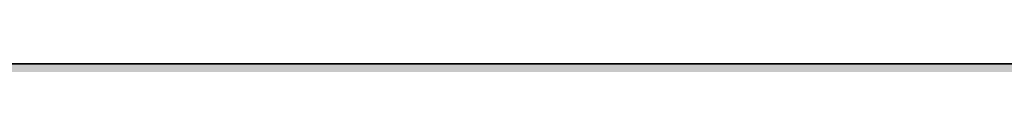
# Model space of a CAD drawing. Units: inches. Extents: x 2091 to 2899, y 967 to 2217.
# Tile 67 of 256: x 2212.646 to 2213.3497, y 1099.9191 to 1099.9191. Entities that reach past the tile are written whole.
import ezdxf

# ---------------------------------------------------------------- set-up
doc = ezdxf.new("R2010")
doc.units = ezdxf.units.IN
doc.layers.add('A-WALL-PATT', color=141, linetype='Continuous', lineweight=13, true_color=0xadddf7)
doc.layers.add('L-SITE-WALL', color=7, linetype='Continuous', lineweight=35)

msp = doc.modelspace()

# ---------------------------------------------------------------- hatches: boundary and pattern name
at = {"layer": 'A-WALL-PATT'}
h = msp.add_hatch(color=256, dxfattribs=at)
h.dxf.hatch_style = 1
h.paths.add_polyline_path([(2212.1436, 1941.41906), (2387.6436, 1941.41906), (2387.6436, 1824.41906), (2392.1436, 1824.41906), (2392.1436, 1941.41906), (2609.6436, 1941.41906), (2609.6436, 1825.91906), (2614.1436, 1825.91906), (2614.1436, 1941.41906), (2794.1436, 1941.41906), (2794.1436, 1928.76217), (2803.1436, 1928.76217), (2803.1436, 2050.91906), (2203.1436, 2050.91906), (2203.1436, 1900.75786), (2212.1436, 1900.75786)])
h.paths.add_polyline_path([(2212.1436, 1945.91906), (2212.1436, 2041.91906), (2794.1436, 2041.91906), (2794.1436, 1945.91906), (2402.24824, 1945.91906), (2401.10243, 1945.77583), (2398.70243, 1945.77583)], flags=16)
h.paths.add_polyline_path([(2230.22986, 1948.06279), (2227.34986, 1949.50279), (2225.90986, 1951.90279), (2223.98986, 1952.86279), (2223.02986, 1955.26279), (2222.06986, 1959.58279), (2222.06986, 1963.42279), (2223.02986, 1965.66279), (2223.98986, 1965.34279), (2225.58591, 1963.86075), (2226.91153, 1964.95726), (2226.94886, 1965.93879), (2227.77832, 1966.95214), (2228.19992, 1968.8787), (2230.70986, 1964.86279), (2233.58986, 1966.30279), (2233.60731, 1966.33187), (2233.77266, 1964.9382), (2234.6338, 1963.67647), (2235.02986, 1963.90279), (2236.28203, 1965.57236), (2235.98986, 1962.94279), (2237.95451, 1957.54), (2238.38986, 1957.90279), (2239.21586, 1960.30579), (2238.65457, 1966.38496), (2238.69279, 1966.43807), (2238.84058, 1967.49971), (2238.78029, 1967.68749), (2238.88054, 1967.78676), (2238.66686, 1966.25179), (2239.21586, 1960.30579), (2238.38986, 1957.90279), (2236.94986, 1956.70279), (2234.54986, 1949.98279)], flags=0)
h.paths.add_polyline_path([(2278.01197, 1948.06279), (2276.49643, 1947.87335), (2275.84983, 1947.68861), (2274.65197, 1947.10279)], flags=0)
h.paths.add_polyline_path([(2269.85197, 1955.74279), (2268.27618, 1956.62933), (2270.8673, 1956.3484), (2269.37197, 1958.14279), (2268.71496, 1959.19233), (2270.56983, 1958.72861), (2268.58073, 1961.90609), (2270.81197, 1960.89188), (2270.81197, 1963.42279), (2271.39331, 1964.77926), (2270.29176, 1966.1562), (2271.77197, 1965.66279), (2272.14139, 1966.52476), (2273.92983, 1965.92861), (2275.63039, 1968.0543), (2276.33194, 1966.72186), (2276.52043, 1966.95214), (2276.94203, 1968.8787), (2277.73429, 1967.61108), (2278.13989, 1969.46452), (2279.65912, 1967.03374), (2280.41197, 1966.78279), (2280.9493, 1967.58879), (2281.60983, 1967.36861), (2282.13327, 1968.15376), (2282.34924, 1966.33344), (2282.34985, 1966.33259), (2283.40755, 1968.09542), (2283.71263, 1965.52402), (2284.32022, 1964.63379), (2284.51181, 1964.88924), (2284.23497, 1965.70479), (2284.50047, 1967.31896), (2284.90794, 1965.41742), (2285.39631, 1966.06858), (2285.43283, 1966.29061), (2285.47334, 1966.17128), (2286.35392, 1967.34539), (2286.22201, 1966.15817), (2287.66349, 1968.08015), (2287.71397, 1968.44279), (2288.4816, 1969.01668), (2288.57399, 1968.7289), (2288.91746, 1969.06904), (2288.60683, 1966.83761), (2288.92873, 1963.35131), (2288.93497, 1963.35679), (2288.92973, 1963.34042), (2289.01528, 1962.41387), (2290.11122, 1963.87513), (2290.13283, 1963.94261), (2290.21767, 1964.01706), (2290.11122, 1963.87513), (2289.15583, 1960.89161), (2288.59404, 1959.25723), (2288.57197, 1959.10279), (2289.53197, 1960.54279), (2290.01197, 1962.46279), (2290.19184, 1962.64266), (2289.76983, 1959.68861), (2286.88983, 1957.28861), (2284.48983, 1950.56861), (2283.31466, 1950.04631), (2283.29197, 1949.98279), (2280.29006, 1948.64861), (2281.12983, 1948.64861), (2282.56983, 1948.16861), (2283.20473, 1948.06279), (2278.97197, 1948.06279), (2276.09197, 1949.50279), (2274.65197, 1951.90279), (2272.73197, 1952.86279)], flags=0)
h.paths.add_polyline_path([(2271.15887, 1958.02177), (2272.96983, 1955.84861), (2272.00983, 1960.16861), (2272.00983, 1964.00861), (2272.62443, 1965.44266), (2274.32802, 1963.86075), (2275.65365, 1964.95726), (2275.63774, 1964.53909), (2277.41223, 1966.00689), (2277.03297, 1965.15679), (2276.82992, 1964.9756), (2276.76601, 1963.29501), (2277.44964, 1962.66022), (2279.45197, 1964.86279), (2282.33197, 1966.30279), (2283.52983, 1966.88861), (2283.29451, 1966.77095), (2283.91299, 1963.8847), (2284.89925, 1964.44827), (2284.73197, 1962.94279), (2286.69662, 1957.54), (2287.13197, 1957.90279), (2287.54191, 1959.09539), (2287.7794, 1958.44231), (2285.68274, 1956.6951), (2285.8765, 1959.79534), (2284.73197, 1962.94279), (2284.89925, 1964.44827), (2283.91299, 1963.8847), (2284.22383, 1962.43412), (2283.42436, 1963.60548), (2281.60983, 1962.56861), (2281.12983, 1960.16861), (2282.08983, 1956.32861), (2283.04983, 1952.96861), (2282.56983, 1950.56861), (2280.16983, 1948.64861), (2279.88332, 1948.79187), (2278.97197, 1948.06279), (2278.97197, 1949.02279), (2278.67231, 1949.39737), (2277.28983, 1950.08861), (2275.84983, 1952.48861), (2273.92983, 1953.44861), (2272.48983, 1954.88861), (2271.92165, 1954.88861), (2271.77197, 1955.26279)], flags=0)
h.paths.add_polyline_path([(2311.99415, 1955.74279), (2312.06272, 1955.67422), (2312.0551, 1955.7085)], flags=0)
h.paths.add_polyline_path([(2331.95615, 1963.95179), (2333.39615, 1965.39179), (2331.07715, 1963.35679), (2330.9986, 1963.11152)], flags=0)
h.paths.add_polyline_path([(2310.55415, 1954.30279), (2307.03981, 1956.27994), (2310.7629, 1955.87628), (2312.47415, 1953.82279), (2313.43415, 1951.42279), (2315.35415, 1950.46279), (2316.79415, 1948.06279), (2317.46615, 1947.72679), (2319.36869, 1947.96461), (2317.75415, 1949.98279), (2317.56953, 1950.61048), (2316.79415, 1951.90279), (2314.87415, 1952.86279), (2313.91415, 1955.26279), (2311.51415, 1958.14279), (2309.37549, 1961.55917), (2311.51415, 1960.33708), (2311.51415, 1961.98279), (2310.60467, 1963.11963), (2311.72661, 1962.47853), (2312.41833, 1964.09256), (2312.25596, 1964.29552), (2313.19415, 1963.98279), (2313.91415, 1965.66279), (2314.64678, 1965.41858), (2315.35415, 1966.30279), (2316.79415, 1967.74279), (2316.15744, 1966.9469), (2317.03411, 1965.28186), (2317.2226, 1965.51214), (2317.77705, 1968.04577), (2318.47411, 1966.72186), (2318.6626, 1966.95214), (2319.0842, 1968.8787), (2321.20705, 1965.48215), (2322.16142, 1966.9137), (2322.55415, 1966.78279), (2322.78599, 1967.13056), (2322.88165, 1966.32429), (2323.31204, 1965.72174), (2323.65129, 1965.89136), (2324.3965, 1967.13338), (2324.65694, 1964.9382), (2324.97199, 1964.47661), (2325.38728, 1967.0015), (2325.94081, 1964.41835), (2327.22893, 1966.13584), (2327.16632, 1965.57236), (2328.05914, 1966.76278), (2328.22458, 1966.24749), (2329.66797, 1967.67691), (2329.66458, 1967.68749), (2329.76482, 1967.78676), (2329.55115, 1966.25179), (2330.10015, 1960.30579), (2329.33281, 1958.07347), (2329.31306, 1957.93523), (2329.63415, 1958.20279), (2330.23415, 1959.10279), (2330.71415, 1961.02279), (2331.03415, 1961.34279), (2330.71415, 1959.10279), (2329.63415, 1958.20279), (2329.27415, 1957.66279), (2327.71211, 1956.3611), (2325.43415, 1949.98279), (2324.33377, 1949.49374), (2323.99415, 1948.54279), (2319.67415, 1946.62279), (2316.79415, 1948.06279), (2315.35415, 1950.46279), (2313.43415, 1951.42279)], flags=0)
h.paths.add_polyline_path([(2321.33568, 1947.95202), (2321.11415, 1948.06279), (2321.11415, 1949.02279), (2319.19415, 1951.42279), (2316.79415, 1959.58279), (2316.66324, 1959.58279), (2315.35415, 1958.14279), (2314.39415, 1958.14279), (2313.1483, 1958.70908), (2312.95415, 1959.58279), (2312.95415, 1960.89188), (2315.83415, 1959.58279), (2316.66324, 1959.58279), (2317.31471, 1960.29941), (2315.0302, 1962.42075), (2316.35582, 1963.51726), (2316.37234, 1963.95162), (2316.4702, 1963.86075), (2317.79582, 1964.95726), (2317.75522, 1963.88969), (2319.17515, 1965.15679), (2319.49841, 1965.88137), (2321.11415, 1965.34279), (2323.23589, 1962.37236), (2325.68635, 1963.77262), (2325.54279, 1962.48058), (2325.19878, 1963.49401), (2324.47851, 1963.08243), (2324.92601, 1960.99412), (2324.07809, 1962.23647), (2322.41479, 1961.28602), (2322.07415, 1959.58279), (2323.03415, 1955.74279), (2323.99415, 1952.38279), (2323.51415, 1949.98279), (2322.14272, 1948.88565), (2322.07415, 1948.54279)], flags=0)
h.paths.add_polyline_path([(2320.20748, 1963.33746), (2320.15415, 1963.42279), (2320.39415, 1963.54279)], flags=0)
h.paths.add_polyline_path([(2353.85053, 1965.8105), (2354.03053, 1965.7505), (2354.33053, 1966.4505), (2354.33053, 1966.9305)], flags=0)
h.paths.add_polyline_path([(2359.02058, 1969.02641), (2359.09838, 1968.90193), (2359.23353, 1969.5195), (2359.23353, 1969.9995)], flags=0)
h.paths.add_polyline_path([(2358.25669, 1966.68167), (2357.9836, 1966.34803), (2358.21127, 1966.14617), (2358.41049, 1966.38957)], flags=0)
h.paths.add_polyline_path([(2357.76847, 1966.05878), (2357.7322, 1965.10497), (2357.75105, 1965.12056), (2357.76953, 1965.6065), (2357.76953, 1966.05784)], flags=0)
h.paths.add_polyline_path([(2359.11153, 1965.3045), (2359.11153, 1964.8245), (2359.84453, 1966.4675), (2359.84453, 1966.9475)], flags=0)
h.paths.add_polyline_path([(2360.22368, 1966.62145), (2360.69853, 1969.3625), (2360.69853, 1969.8425), (2360.21053, 1967.0255), (2360.21053, 1966.6425)], flags=0)
h.paths.add_polyline_path([(2363.45053, 1967.8905), (2363.45053, 1968.3705), (2362.49053, 1966.9305), (2362.65604, 1966.69878)], flags=0)
h.paths.add_polyline_path([(2364.47552, 1966.07883), (2365.85053, 1968.3705), (2365.85053, 1968.8505), (2364.42798, 1966.47958)], flags=0)
h.paths.add_polyline_path([(2366.31353, 1965.8525), (2366.36671, 1965.69583), (2366.80253, 1968.3455), (2366.80253, 1968.8255)], flags=0)
h.paths.add_polyline_path([(2367.16531, 1965.80354), (2367.29053, 1966.9305), (2367.29053, 1967.4105), (2367.1027, 1965.72007)], flags=0)
h.paths.add_polyline_path([(2370.03653, 1959.9735), (2371.01353, 1963.0245), (2371.01353, 1963.5045), (2370.03653, 1960.4535)], flags=0)
h.paths.add_polyline_path([(2371.61053, 1960.2105), (2372.57053, 1961.6505), (2372.57053, 1962.1305), (2371.80253, 1960.9785)], flags=0)
h.paths.add_polyline_path([(2350.87367, 1956.00509), (2351.93053, 1955.8905), (2354.49053, 1953.3305), (2353.85053, 1954.9305), (2351.45053, 1957.8105), (2347.93553, 1963.4255), (2347.93553, 1963.9055), (2351.45053, 1958.2905), (2353.70507, 1955.58505), (2352.89053, 1959.2505), (2352.89053, 1959.7305), (2352.89053, 1961.92479), (2356.73053, 1959.7305), (2358.45447, 1961.62684), (2354.81053, 1965.0105), (2355.03086, 1965.28591), (2358.69109, 1961.88712), (2361.53053, 1965.0105), (2364.3765, 1966.43348), (2364.52439, 1965.18691), (2365.45447, 1963.82418), (2365.88107, 1964.06795), (2365.37053, 1966.4505), (2365.37053, 1966.9305), (2366.81053, 1960.2105), (2366.81053, 1959.7305), (2366.38871, 1952.98141), (2367.77053, 1956.8505), (2368.64123, 1957.57608), (2366.81053, 1962.6105), (2366.81053, 1963.0905), (2368.77518, 1957.68771), (2369.21053, 1958.0505), (2370.00159, 1960.35187), (2369.47523, 1966.05267), (2369.51346, 1966.10578), (2369.51417, 1966.11091), (2369.47523, 1966.53267), (2369.51346, 1966.58578), (2369.61463, 1967.31259), (2369.18253, 1968.6585), (2369.18253, 1969.1385), (2369.60096, 1967.83519), (2369.7012, 1967.93447), (2369.71795, 1968.05474), (2370.14518, 1968.37414), (2369.77871, 1968.01122), (2369.7012, 1967.45447), (2370.46816, 1968.214), (2369.67494, 1967.26577), (2369.51417, 1966.11091), (2370.03653, 1960.4535), (2370.03653, 1959.9735), (2369.44176, 1958.24319), (2370.65053, 1959.2505), (2371.04582, 1962.01756), (2371.13053, 1962.1305), (2370.65053, 1958.7705), (2367.77053, 1956.3705), (2365.37053, 1949.6505), (2362.0791, 1948.18764), (2363.45053, 1947.7305), (2361.05053, 1947.7305), (2360.09053, 1947.7305), (2357.10386, 1947.35717), (2360.09053, 1948.2105), (2358.17053, 1949.1705), (2356.73053, 1951.5705), (2354.81053, 1952.5305), (2351.93053, 1955.4105)], flags=0)
h.paths.add_polyline_path([(2361.05053, 1948.6905), (2359.13053, 1951.0905), (2356.73053, 1959.2505), (2355.77053, 1959.2505), (2352.89053, 1960.55959), (2352.89053, 1961.44479), (2355.89053, 1959.7305), (2356.73053, 1959.7305), (2356.83719, 1959.36783), (2361.53053, 1964.5305), (2363.24842, 1965.38945), (2364.92531, 1963.0418), (2362.49053, 1961.6505), (2362.06386, 1959.51717), (2362.97053, 1955.8905), (2363.93053, 1952.5305), (2363.93053, 1952.0505), (2363.45053, 1949.6505), (2361.05053, 1947.7305)], flags=0)
h.paths.add_polyline_path([(2359.13053, 1951.5705), (2359.29053, 1951.3705), (2361.05053, 1954.4505), (2361.05053, 1954.9305)], flags=0)
h.paths.add_polyline_path([(2357.21953, 1966.5455), (2356.79253, 1968.8145), (2356.79253, 1969.2945), (2357.21953, 1967.0255)], flags=0)
h.paths.add_polyline_path([(2361.05053, 1954.4505), (2361.53053, 1958.7705), (2361.53053, 1959.2505), (2361.05053, 1954.9305)], flags=0)
h.paths.add_polyline_path([(2402.54829, 1948.48608), (2402.30243, 1948.41583), (2402.59043, 1948.41583)], flags=0)
h.paths.add_polyline_path([(2394.14243, 1956.09583), (2395.68505, 1954.55321), (2396.7205, 1953.97068), (2396.06243, 1955.61583), (2395.24138, 1956.6011), (2395.8789, 1956.44171), (2395.10243, 1959.93583), (2395.10243, 1963.77583), (2396.06243, 1966.01583), (2397.02243, 1965.69583), (2398.61848, 1964.21379), (2399.94411, 1965.3103), (2399.98143, 1966.29183), (2400.81089, 1967.30518), (2401.23249, 1969.23174), (2403.53795, 1965.54301), (2403.94198, 1967.38932), (2404.70243, 1967.13583), (2405.46033, 1966.07478), (2406.62243, 1966.65583), (2406.63988, 1966.68491), (2406.80523, 1965.29124), (2406.92569, 1965.11475), (2407.34243, 1964.97583), (2407.87433, 1965.77367), (2408.1691, 1964.39805), (2409.31461, 1965.9254), (2409.21746, 1965.05105), (2409.44523, 1963.13124), (2410.30637, 1961.86951), (2410.70243, 1962.09583), (2411.44227, 1963.08228), (2411.16543, 1963.89783), (2411.61643, 1966.63976), (2411.72536, 1966.79111), (2411.87315, 1967.85275), (2411.81286, 1968.04053), (2411.91311, 1968.1398), (2411.69943, 1966.60483), (2412.24843, 1960.65883), (2413.22543, 1963.70983), (2414.3779, 1964.72116), (2414.51315, 1965.69275), (2414.45286, 1965.88053), (2414.55311, 1965.9798), (2414.3779, 1964.72116), (2414.51982, 1964.8457), (2414.36536, 1964.63111), (2414.33943, 1964.44483), (2414.88843, 1958.49883), (2414.06243, 1956.09583), (2412.62243, 1954.89583), (2410.17137, 1948.03285), (2410.01672, 1948.0844), (2405.90243, 1946.25583), (2405.90243, 1947.21583), (2405.20425, 1948.08856), (2404.22243, 1948.41583), (2403.26243, 1948.41583), (2400.38243, 1949.85583), (2399.66243, 1951.05583), (2397.98243, 1952.73583), (2397.02243, 1953.21583), (2395.68505, 1954.55321), (2392.65678, 1956.25691)], flags=0)
h.paths.add_polyline_path([(2409.08565, 1964.40744), (2409.13036, 1964.27572), (2409.26243, 1964.49583)], flags=0)
h.paths.add_polyline_path([(2397.74243, 1961.61583), (2398.70243, 1963.85583), (2399.66243, 1963.53583), (2401.42656, 1965.74099), (2401.79142, 1966.5588), (2402.07143, 1965.07083), (2402.83551, 1964.39337), (2403.2624, 1964.9149), (2403.33812, 1964.77109), (2402.61552, 1963.97622), (2402.49861, 1960.90224), (2403.543, 1959.93245), (2404.4132, 1960.88968), (2404.70243, 1962.33583), (2407.91635, 1964.17235), (2409.52021, 1961.92694), (2410.98708, 1957.89304), (2411.42243, 1958.25583), (2412.04796, 1960.07562), (2412.41034, 1959.07909), (2411.67562, 1958.46682), (2411.66243, 1958.25583), (2411.62607, 1958.42553), (2409.98243, 1957.05583), (2407.58243, 1950.33583), (2403.26243, 1948.41583), (2403.26243, 1949.37583), (2401.34243, 1951.77583), (2399.41651, 1958.32398), (2397.74243, 1959.08492), (2397.74243, 1959.97012), (2397.10243, 1960.33583), (2397.74243, 1960.04492)], flags=0)
h.paths.add_polyline_path([(2405.90243, 1952.97583), (2405.95043, 1953.40783), (2406.01672, 1953.17583)], flags=0)
h.paths.add_polyline_path([(2449.81778, 1967.11401), (2449.75232, 1967.13583), (2449.7937, 1967.0779)], flags=0)
h.paths.add_polyline_path([(2451.6977, 1966.61812), (2451.74089, 1966.69012), (2451.69205, 1966.6657)], flags=0)
h.paths.add_polyline_path([(2454.34363, 1965.73757), (2455.75232, 1967.61583), (2455.99232, 1968.09583), (2454.3645, 1965.9254)], flags=0)
h.paths.add_polyline_path([(2457.54732, 1968.86383), (2457.78732, 1969.34383), (2457.05432, 1968.79583), (2457.00762, 1968.46034)], flags=0)
h.paths.add_polyline_path([(2456.92178, 1967.85666), (2456.80224, 1968.22902), (2456.723, 1967.6598)], flags=0)
h.paths.add_polyline_path([(2457.30232, 1967.37683), (2457.54232, 1967.85683), (2456.81032, 1966.83983), (2456.74052, 1966.70022), (2456.74902, 1966.60811)], flags=0)
h.paths.add_polyline_path([(2458.27532, 1963.70983), (2458.15534, 1963.33515), (2460.35432, 1965.26483), (2460.59432, 1965.74483)], flags=0)
h.paths.add_polyline_path([(2458.39232, 1962.81583), (2458.36409, 1962.61819), (2459.59232, 1964.25583), (2459.83232, 1964.73583)], flags=0)
h.paths.add_polyline_path([(2459.35232, 1962.81583), (2459.27232, 1962.49583), (2460.07232, 1963.29583), (2460.31232, 1963.77583)], flags=0)
h.paths.add_polyline_path([(2458.68032, 1960.60783), (2458.63232, 1960.41583), (2459.59232, 1961.85583), (2459.83232, 1962.33583)], flags=0)
h.paths.add_polyline_path([(2437.83817, 1956.24265), (2439.19232, 1956.09583), (2441.35232, 1953.93583), (2440.87232, 1955.13583), (2438.47232, 1958.01583), (2438.07156, 1958.65602), (2438.71232, 1958.49583), (2440.6396, 1956.18311), (2439.91232, 1959.45583), (2439.91232, 1963.29583), (2441.35232, 1966.65583), (2441.59232, 1967.13583), (2441.11232, 1966.01583), (2442.07232, 1965.69583), (2443.98899, 1968.09167), (2444.24132, 1966.75083), (2444.9168, 1966.15192), (2445.67657, 1967.08014), (2446.25532, 1969.72483), (2446.49532, 1970.20483), (2446.28238, 1969.23174), (2447.36267, 1967.50327), (2447.72032, 1969.56783), (2447.96032, 1970.04783), (2447.48548, 1967.30678), (2448.79232, 1965.21583), (2448.47232, 1964.86383), (2448.55232, 1964.73583), (2451.45205, 1966.1857), (2451.61512, 1964.81124), (2452.30792, 1963.79617), (2453.23451, 1964.32565), (2454.07232, 1960.41583), (2453.62869, 1953.31765), (2454.79232, 1956.57583), (2455.03232, 1957.05583), (2455.71884, 1957.62793), (2453.83232, 1962.81583), (2453.94097, 1963.79362), (2453.33532, 1965.57783), (2453.82432, 1968.55083), (2454.06432, 1969.03083), (2453.57532, 1966.05783), (2454.04033, 1964.68792), (2453.83232, 1962.81583), (2455.71884, 1957.62793), (2456.36721, 1958.16824), (2457.05832, 1960.17883), (2457.29832, 1960.65883), (2456.47232, 1958.25583), (2457.71773, 1959.29367), (2457.67232, 1958.97583), (2454.88995, 1956.65719), (2453.61414, 1953.08492), (2453.59232, 1952.73583), (2453.35232, 1952.25583), (2453.3596, 1952.3722), (2452.63232, 1950.33583), (2452.39232, 1949.85583), (2449.20375, 1948.43869), (2450.71232, 1947.93583), (2448.07232, 1947.93583), (2447.11232, 1947.93583), (2444.55232, 1947.61583), (2447.1996, 1948.3722), (2445.19232, 1949.37583), (2443.75232, 1951.77583), (2441.83232, 1952.73583), (2438.95232, 1955.61583)], flags=0)
h.paths.add_polyline_path([(2443.99232, 1959.93583), (2444.04032, 1959.77263), (2444.12155, 1959.86199)], flags=0)
h.paths.add_polyline_path([(2442.91232, 1959.93583), (2443.03232, 1959.93583), (2442.44566, 1960.2025)], flags=0)
h.paths.add_polyline_path([(2444.98294, 1965.01968), (2445.27932, 1965.26483), (2445.51932, 1965.74483), (2444.994, 1965.3103)], flags=0)
h.paths.add_polyline_path([(2446.13332, 1965.02983), (2446.33037, 1965.4715), (2444.97032, 1964.25783), (2444.73032, 1963.77783)], flags=0)
h.paths.add_polyline_path([(2442.79232, 1959.45583), (2443.75232, 1959.45583), (2446.15232, 1951.29583), (2446.41232, 1951.75083), (2446.39232, 1951.77583), (2448.0806, 1954.73032), (2448.55232, 1958.97583), (2441.83232, 1965.21583), (2442.15495, 1965.61911), (2448.79232, 1959.45583), (2448.31232, 1955.13583), (2448.07232, 1954.65583), (2446.41232, 1951.75083), (2448.31232, 1949.37583), (2448.31232, 1948.41583), (2450.54089, 1950.19869), (2450.95232, 1952.25583), (2449.99232, 1955.61583), (2449.03232, 1959.45583), (2449.51232, 1961.85583), (2449.75232, 1962.33583), (2449.6749, 1961.94874), (2452.99451, 1963.84565), (2453.06441, 1963.51941), (2452.88461, 1963.78285), (2449.6749, 1961.94874), (2449.27232, 1959.93583), (2450.23232, 1956.09583), (2451.19232, 1952.73583), (2450.71232, 1950.33583), (2450.47232, 1949.85583), (2448.07232, 1947.93583), (2448.07232, 1948.53583), (2445.43232, 1949.85583), (2443.99232, 1952.25583), (2442.07232, 1953.21583), (2441.11232, 1955.61583), (2440.15232, 1959.93583), (2440.15232, 1960.65583)], flags=0)
h.paths.add_polyline_path([(2456.69232, 1966.98583), (2457.60832, 1968.08083), (2457.84832, 1968.56083), (2456.93232, 1967.46583)], flags=0)
h.paths.add_polyline_path([(2489.89657, 1966.58024), (2489.94295, 1966.18935), (2490.74749, 1967.53025), (2491.31912, 1968.95116)], flags=0)
h.paths.add_polyline_path([(2473.56247, 1956.40713), (2477.13998, 1956.01926), (2476.95533, 1956.24083), (2475.10805, 1957.28011), (2476.34749, 1956.97025), (2475.1869, 1958.82422), (2476.91912, 1958.39116), (2475.41164, 1960.79927), (2477.78749, 1959.71934), (2477.78749, 1962.25025), (2477.6374, 1962.43786), (2477.82255, 1962.33206), (2478.35912, 1963.58406), (2478.35912, 1963.67116), (2477.32435, 1964.96463), (2478.71483, 1964.50114), (2479.31912, 1965.91116), (2480.27912, 1965.59116), (2481.78397, 1967.47221), (2482.11649, 1965.70525), (2482.88056, 1965.02778), (2483.20931, 1965.42941), (2483.22017, 1965.71509), (2483.07594, 1965.98902), (2483.71176, 1966.76581), (2484.13049, 1968.67925), (2484.70212, 1970.10016), (2484.48918, 1969.12707), (2486.5029, 1965.90511), (2487.38749, 1965.61025), (2488.15342, 1966.75914), (2488.71702, 1965.97011), (2489.20009, 1966.21164), (2489.33067, 1965.11099), (2490.3939, 1963.62246), (2490.66077, 1963.77496), (2490.49391, 1964.55364), (2490.92306, 1963.92484), (2491.31912, 1964.15116), (2491.33339, 1964.17018), (2491.21049, 1964.53225), (2491.28176, 1964.96554), (2491.42579, 1964.29338), (2494.07648, 1967.82763), (2494.49792, 1966.51494), (2494.59817, 1966.61422), (2494.68949, 1967.27025), (2495.10675, 1967.5822), (2495.12984, 1967.74807), (2495.06955, 1967.93585), (2495.1698, 1968.03513), (2495.03178, 1967.04363), (2495.75382, 1967.75868), (2494.98205, 1966.68644), (2494.95612, 1966.50016), (2495.47902, 1960.83685), (2495.91049, 1962.18425), (2496.48212, 1963.60516), (2496.07269, 1962.32659), (2496.7689, 1962.93754), (2496.59912, 1962.71116), (2496.11912, 1959.35116), (2496.73287, 1960.27179), (2496.98749, 1961.29025), (2497.55912, 1962.71116), (2497.07912, 1960.79116), (2496.50749, 1959.37025), (2495.54749, 1957.93025), (2492.75884, 1955.60638), (2490.83912, 1950.23116), (2490.26749, 1948.81025), (2485.94749, 1946.89025), (2483.06749, 1948.33025), (2481.62749, 1950.73025), (2479.70749, 1951.69025), (2476.82749, 1954.57025)], flags=0)
h.paths.add_polyline_path([(2485.57697, 1948.31339), (2485.55912, 1948.31116), (2485.57876, 1948.31116)], flags=0)
h.paths.add_polyline_path([(2478.64506, 1954.55116), (2478.10904, 1956.96326), (2479.31912, 1955.51116), (2480.27912, 1953.11116), (2482.19912, 1952.15116), (2483.63912, 1949.75116), (2486.51912, 1948.31116), (2486.51912, 1949.27116), (2484.73931, 1951.49593), (2484.02749, 1950.25025), (2481.62749, 1958.41025), (2482.37515, 1959.23267), (2482.19912, 1959.83116), (2483.19757, 1960.92946), (2479.70749, 1964.17025), (2480.60336, 1965.29008), (2481.87517, 1964.10911), (2482.66639, 1964.76358), (2482.61536, 1963.4218), (2482.9892, 1963.07466), (2484.00849, 1963.98425), (2484.68361, 1965.49751), (2484.58012, 1965.40516), (2485.35727, 1967.14711), (2485.12065, 1965.7812), (2486.42749, 1963.69025), (2488.14538, 1964.5492), (2489.82227, 1962.20155), (2490.74749, 1962.73025), (2491.99966, 1964.39981), (2492.07605, 1965.08726), (2492.21289, 1964.68412), (2492.48537, 1965.04743), (2492.27912, 1963.19116), (2494.24377, 1957.78837), (2494.5625, 1958.05398), (2494.93349, 1959.13325), (2495.50512, 1960.55416), (2494.67912, 1958.15116), (2494.10749, 1956.73025), (2494.5625, 1958.05398), (2493.40854, 1957.09235), (2491.70749, 1961.77025), (2491.99966, 1964.39981), (2490.74749, 1962.73025), (2487.71203, 1960.9957), (2487.47912, 1959.83116), (2488.43912, 1955.99116), (2489.39912, 1952.63116), (2488.91912, 1950.23116), (2488.57692, 1949.9574), (2488.34749, 1948.81025), (2487.65172, 1948.25363), (2487.47912, 1948.31116), (2486.51912, 1948.31116), (2483.63912, 1949.75116), (2482.19912, 1952.15116), (2480.27912, 1953.11116), (2478.83912, 1954.55116)], flags=0)
h.paths.add_polyline_path([(2526.64825, 1966.98752), (2526.51734, 1967.03116), (2526.6001, 1966.9153)], flags=0)
h.paths.add_polyline_path([(2528.47064, 1966.44666), (2528.57449, 1966.61973), (2528.45707, 1966.56102)], flags=0)
h.paths.add_polyline_path([(2534.13334, 1967.49616), (2534.15669, 1967.54285), (2534.05984, 1967.4083)], flags=0)
h.paths.add_polyline_path([(2536.16192, 1964.0506), (2535.15734, 1962.71116), (2535.10087, 1962.31587), (2536.11734, 1963.67116), (2536.42053, 1964.27754)], flags=0)
h.paths.add_polyline_path([(2535.15734, 1959.83116), (2536.11734, 1961.27116), (2536.59734, 1962.23116), (2535.25334, 1960.21516)], flags=0)
h.paths.add_polyline_path([(2513.24904, 1956.2848), (2516.22118, 1955.96256), (2514.99734, 1957.43116), (2514.19582, 1958.71154), (2515.47734, 1958.39116), (2516.93189, 1956.64571), (2516.43734, 1958.87116), (2516.43734, 1962.71116), (2516.87269, 1963.72697), (2515.34643, 1965.6348), (2517.39734, 1964.95116), (2517.87734, 1966.07116), (2518.35734, 1967.03116), (2517.87734, 1965.91116), (2518.83734, 1965.59116), (2520.48659, 1967.65272), (2520.76634, 1966.16616), (2521.53042, 1965.48869), (2521.78144, 1965.79537), (2521.80091, 1966.30727), (2521.4778, 1966.92094), (2521.24634, 1967.12616), (2521.1777, 1967.49091), (2521.4778, 1966.92094), (2522.01042, 1966.44869), (2522.25739, 1966.75042), (2522.78034, 1969.14016), (2523.26034, 1970.10016), (2523.0474, 1969.12707), (2524.67313, 1966.5259), (2526.03734, 1966.07116), (2526.79524, 1965.01011), (2527.97707, 1965.60102), (2528.14014, 1964.22657), (2528.66459, 1963.45816), (2529.38862, 1963.87189), (2529.32967, 1964.14699), (2529.48128, 1963.92484), (2529.87734, 1964.15116), (2529.98401, 1964.29338), (2529.78905, 1965.20318), (2530.0624, 1964.3979), (2532.80248, 1968.05135), (2533.14777, 1966.97585), (2533.24802, 1967.07513), (2533.33934, 1967.73116), (2533.67285, 1967.98049), (2533.72802, 1968.03513), (2533.51434, 1966.50016), (2534.02472, 1960.9725), (2534.56034, 1962.64516), (2535.04034, 1963.60516), (2534.06334, 1960.55416), (2533.23734, 1958.15116), (2534.28815, 1959.02684), (2534.19734, 1958.39116), (2531.5126, 1956.15387), (2529.39734, 1950.23116), (2528.91734, 1949.27116), (2526.44877, 1948.17402), (2527.47734, 1947.83116), (2530.35734, 1947.35116), (2524.59734, 1947.35116), (2521.71734, 1948.79116), (2520.27734, 1951.19116), (2518.35734, 1952.15116), (2515.47734, 1955.03116)], flags=0)
h.paths.add_polyline_path([(2523.93476, 1967.19031), (2523.61951, 1966.48369), (2523.7705, 1966.24211)], flags=0)
h.paths.add_polyline_path([(2518.83734, 1953.11116), (2517.87734, 1955.51116), (2516.88498, 1959.97678), (2516.91734, 1959.96207), (2516.91734, 1962.02545), (2520.75734, 1959.83116), (2522.02495, 1961.22553), (2518.35734, 1964.63116), (2519.00259, 1965.43772), (2520.43339, 1964.10911), (2521.30112, 1964.82687), (2521.24516, 1963.35533), (2525.63831, 1959.27598), (2526.03734, 1961.27116), (2529.39734, 1963.19116), (2530.64952, 1964.86073), (2530.66472, 1964.99755), (2530.69196, 1964.91731), (2531.08778, 1965.44507), (2530.94599, 1964.16894), (2530.69196, 1964.91731), (2529.39734, 1963.19116), (2526.3625, 1961.45697), (2526.03734, 1959.83116), (2526.99734, 1955.99116), (2527.95734, 1952.63116), (2527.47734, 1950.23116), (2527.13449, 1949.95687), (2526.97393, 1949.15409), (2526.69734, 1949.03116), (2524.59734, 1947.35116), (2524.59734, 1948.31116), (2524.27734, 1948.71116), (2522.19734, 1949.75116), (2520.75734, 1952.15116)], flags=0)
h.paths.add_polyline_path([(2520.27734, 1958.87116), (2520.85334, 1959.50476), (2523.15734, 1951.67116), (2524.61389, 1954.22013), (2524.59734, 1954.07116), (2522.67734, 1950.71116)], flags=0)
h.paths.add_polyline_path([(2559.37091, 1966.31116), (2559.39841, 1966.32491), (2559.40194, 1966.3453)], flags=0)
h.paths.add_polyline_path([(2549.77091, 1957.19116), (2552.65091, 1954.31116), (2552.13399, 1955.60347), (2550.61091, 1957.43116), (2547.09591, 1963.04616), (2545.77591, 1965.20616), (2549.29091, 1959.59116), (2551.69091, 1956.71116), (2550.79293, 1960.75206), (2550.73091, 1960.78025), (2550.73091, 1964.87116), (2551.69091, 1967.11116), (2552.65091, 1966.79116), (2554.24696, 1965.30911), (2555.03425, 1965.96034), (2555.58167, 1966.64461), (2555.60991, 1967.38716), (2556.43937, 1968.40051), (2556.86097, 1970.32707), (2559.37091, 1966.31116), (2560.69091, 1964.15116), (2562.40881, 1965.01011), (2561.65091, 1966.07116), (2560.33091, 1968.23116), (2561.7585, 1966.23254), (2562.34721, 1967.11561), (2562.43371, 1966.38657), (2563.1278, 1965.3696), (2563.57091, 1965.59116), (2563.58836, 1965.62024), (2563.36254, 1967.52354), (2563.72249, 1965.84379), (2565.06, 1968.07298), (2564.73286, 1965.12872), (2565.11758, 1963.33338), (2567.44462, 1966.43611), (2567.31561, 1967.83333), (2567.35384, 1967.88644), (2567.50163, 1968.94807), (2567.44134, 1969.13585), (2567.54159, 1969.23513), (2567.32791, 1967.70016), (2567.87691, 1961.75416), (2568.74669, 1964.47033), (2568.63561, 1965.67333), (2568.67384, 1965.72644), (2568.82163, 1966.78807), (2568.76134, 1966.97585), (2568.86159, 1967.07513), (2568.64791, 1965.54016), (2568.72613, 1964.69303), (2568.85391, 1964.80516), (2568.74669, 1964.47033), (2568.81724, 1963.70626), (2568.97091, 1963.91116), (2568.86607, 1963.17731), (2569.19691, 1959.59416), (2568.37091, 1957.19116), (2566.93091, 1955.99116), (2564.62027, 1949.52137), (2564.65091, 1949.51116), (2564.61662, 1949.51116), (2564.53091, 1949.27116), (2560.21091, 1947.35116), (2557.33091, 1948.79116), (2556.0452, 1950.93402), (2556.01091, 1950.95116), (2555.85662, 1951.2083), (2553.97091, 1952.15116), (2551.09091, 1955.03116), (2546.65014, 1957.52951)], flags=0)
h.paths.add_polyline_path([(2567.02579, 1959.33023), (2567.03501, 1959.30489), (2567.05091, 1959.35116)], flags=0)
h.paths.add_polyline_path([(2551.96829, 1962.51837), (2553.01091, 1964.95116), (2553.97091, 1964.63116), (2555.56696, 1963.14911), (2556.89258, 1964.24563), (2556.92991, 1965.22716), (2557.14398, 1965.48869), (2556.42007, 1966.13056), (2556.39142, 1966.10499), (2556.37991, 1966.16616), (2556.42007, 1966.13056), (2556.95191, 1966.60516), (2557.09214, 1966.91948), (2557.57087, 1966.01023), (2557.75937, 1966.24051), (2557.41791, 1964.68016), (2556.89258, 1964.24563), (2556.80709, 1961.99757), (2560.69091, 1958.39116), (2560.63553, 1957.8927), (2560.81091, 1957.19116), (2561.77091, 1953.83116), (2561.29091, 1951.43116), (2559.11042, 1949.68677), (2559.15648, 1949.62919), (2563.02652, 1951.34921), (2562.61091, 1949.27116), (2560.21091, 1947.35116), (2560.21091, 1948.31116), (2559.25091, 1949.51116), (2558.89091, 1949.51116), (2558.89091, 1949.96116), (2558.29091, 1950.71116), (2558.0537, 1951.51767), (2556.97091, 1952.87116), (2555.06788, 1959.34146), (2552.05091, 1961.06545), (2552.05091, 1962.47116)], flags=0)
h.paths.add_polyline_path([(2588.33005, 1958.39116), (2588.61025, 1958.11096), (2588.55336, 1958.36695)], flags=0)
h.paths.add_polyline_path([(2594.74545, 1950.49309), (2593.95753, 1953.17202), (2593.13005, 1954.55116), (2591.21005, 1955.51116), (2590.25005, 1957.91116), (2588.30903, 1960.24038), (2586.17731, 1961.20935), (2587.85005, 1960.79116), (2587.25342, 1961.74425), (2588.44131, 1961.06545), (2588.44131, 1962.65553), (2588.42168, 1962.66535), (2588.44131, 1962.71116), (2586.91404, 1964.62026), (2588.87709, 1963.72796), (2589.29005, 1964.69154), (2589.29005, 1966.07116), (2590.25005, 1968.31116), (2591.21005, 1967.99116), (2592.8061, 1966.50911), (2594.13172, 1967.60563), (2594.16905, 1968.58716), (2594.99851, 1969.60051), (2595.4201, 1971.52707), (2597.93005, 1967.51116), (2600.81005, 1968.95116), (2600.8275, 1968.98024), (2600.99285, 1967.58657), (2601.85399, 1966.32484), (2602.10714, 1966.4695), (2602.23635, 1967.25507), (2602.35672, 1966.69338), (2603.50222, 1968.22073), (2603.21005, 1965.59116), (2605.1747, 1960.18837), (2605.50689, 1960.4652), (2605.02602, 1965.67333), (2605.06425, 1965.72644), (2605.21203, 1966.78807), (2605.15174, 1966.97585), (2605.25199, 1967.07513), (2605.34331, 1967.73116), (2605.9529, 1968.1869), (2605.87475, 1969.03333), (2605.91298, 1969.08644), (2606.06077, 1970.14807), (2606.00048, 1970.33585), (2606.10073, 1970.43513), (2605.88705, 1968.90016), (2606.43605, 1962.95416), (2605.61005, 1960.55116), (2605.99704, 1960.87365), (2606.56431, 1962.64516), (2608.24149, 1964.11694), (2608.01005, 1963.19116), (2607.05005, 1961.75116), (2606.63149, 1961.40236), (2606.20131, 1958.39116), (2603.32131, 1955.99116), (2600.92131, 1949.27116), (2596.60131, 1947.35116), (2593.72131, 1948.79116), (2592.85731, 1950.23116), (2592.65005, 1950.23116)], flags=0)
h.paths.add_polyline_path([(2596.60131, 1947.35116), (2596.60131, 1948.31116), (2594.68131, 1950.71116), (2596.15495, 1953.29003), (2595.53005, 1954.07116), (2593.19923, 1961.99596), (2592.65134, 1962.50471), (2591.78015, 1963.00253), (2593.28299, 1964.24563), (2593.32031, 1965.22716), (2594.14977, 1966.24051), (2594.57137, 1968.16707), (2596.18265, 1965.58902), (2596.95127, 1966.43451), (2598.04131, 1966.07116), (2598.79921, 1965.01011), (2599.96131, 1965.59116), (2599.97876, 1965.62024), (2600.14411, 1964.22657), (2601.00526, 1962.96484), (2601.40131, 1963.19116), (2602.65349, 1964.86073), (2602.36131, 1962.23116), (2603.79275, 1958.29472), (2601.97764, 1953.21243), (2601.94621, 1952.70945), (2599.46876, 1951.60836), (2599.00131, 1949.27116)], flags=0)
h.paths.add_polyline_path([(2597.56131, 1958.87116), (2597.67097, 1959.41942), (2597.59505, 1958.7362)], flags=0)
h.paths.add_polyline_path([(2623.6663, 1961.25438), (2625.51916, 1960.79116), (2624.96554, 1961.67553), (2627.19916, 1960.66025), (2627.19916, 1961.15116), (2626.95916, 1962.23116), (2626.95916, 1963.49116), (2625.58232, 1965.21221), (2626.95916, 1964.42545), (2626.95916, 1965.83116), (2626.86916, 1965.86116), (2627.91916, 1968.31116), (2628.87916, 1967.99116), (2630.47521, 1966.50911), (2631.80084, 1967.60563), (2631.83816, 1968.58716), (2632.66762, 1969.60051), (2633.08922, 1971.52707), (2635.59916, 1967.51116), (2638.47916, 1968.95116), (2638.49661, 1968.98024), (2638.66196, 1967.58657), (2639.17627, 1966.83301), (2639.78022, 1967.83958), (2640.02583, 1966.69338), (2641.17134, 1968.22073), (2640.87916, 1965.59116), (2641.11426, 1964.94463), (2641.41134, 1965.34073), (2641.3081, 1964.41159), (2642.84381, 1960.18837), (2643.27916, 1960.55116), (2644.08474, 1962.89474), (2643.78387, 1966.15333), (2643.80683, 1966.18524), (2643.60068, 1968.41805), (2643.52281, 1968.66058), (2643.72988, 1970.14807), (2643.66959, 1970.33585), (2643.76984, 1970.43513), (2643.55616, 1968.90016), (2643.60068, 1968.41805), (2643.90959, 1967.45585), (2644.00984, 1967.55513), (2643.81174, 1966.13208), (2644.10516, 1962.95416), (2644.23877, 1961.35084), (2644.71916, 1961.75116), (2645.03285, 1962.2217), (2645.32216, 1963.12516), (2646.07642, 1963.78705), (2645.03285, 1962.2217), (2644.34516, 1960.07416), (2643.51916, 1957.67116), (2642.07916, 1956.47116), (2639.71961, 1949.86442), (2639.87553, 1949.83843), (2635.35916, 1947.83116), (2632.47916, 1949.27116), (2631.03916, 1951.67116), (2629.11916, 1952.63116), (2628.15916, 1955.03116), (2625.75916, 1957.91116)], flags=0)
h.paths.add_polyline_path([(2627.81631, 1956.57402), (2627.37371, 1958.56571), (2626.37631, 1959.76259), (2627.19916, 1959.35116), (2627.37371, 1958.56571), (2627.91916, 1957.91116), (2628.87916, 1955.51116), (2630.79916, 1954.55116), (2632.23916, 1952.15116), (2633.31502, 1951.61323), (2631.03916, 1959.35116), (2631.49783, 1959.85569), (2630.79916, 1962.23116), (2631.44987, 1962.94694), (2630.71521, 1963.62911), (2632.04084, 1964.72563), (2632.07816, 1965.70716), (2632.29224, 1965.96869), (2631.70534, 1966.48907), (2633.13644, 1967.76614), (2633.32922, 1968.64707), (2634.67472, 1966.49427), (2635.20847, 1967.08139), (2636.79916, 1966.55116), (2637.6764, 1967.86702), (2638.99395, 1966.02246), (2639.70534, 1966.42898), (2641.11916, 1959.83116), (2640.93007, 1956.80571), (2639.43916, 1952.63116), (2638.22746, 1952.09262), (2637.75916, 1949.75116), (2635.35916, 1947.83116), (2635.35916, 1948.79116), (2633.43916, 1951.19116), (2633.31502, 1951.61323), (2632.23916, 1952.15116), (2630.79916, 1954.55116), (2628.87916, 1955.51116)], flags=0)
h.paths.add_polyline_path([(2637.75916, 1953.83116), (2637.27916, 1955.51116), (2636.31916, 1959.35116), (2636.79916, 1961.75116), (2639.23395, 1963.14246), (2637.55706, 1965.49011), (2638.73889, 1966.08102), (2638.90196, 1964.70657), (2639.7631, 1963.44484), (2636.79916, 1961.75116), (2636.5325, 1960.41783), (2637.03916, 1958.39116), (2637.99916, 1955.03116)], flags=0)
h.paths.add_polyline_path([(2668.56741, 1951.43116), (2667.60741, 1953.83116), (2665.20741, 1956.71116), (2662.2939, 1961.36531), (2665.44741, 1959.59116), (2666.64741, 1958.39116), (2666.64741, 1959.97516), (2666.05832, 1960.68207), (2666.64741, 1960.34545), (2666.64741, 1961.99116), (2666.70009, 1962.11409), (2666.40741, 1963.43116), (2666.40741, 1967.27116), (2667.36741, 1969.51116), (2668.32741, 1969.19116), (2669.92346, 1967.70911), (2671.24908, 1968.80563), (2671.28641, 1969.78716), (2672.11587, 1970.80051), (2672.53746, 1972.72707), (2675.04741, 1968.71116), (2677.92741, 1970.15116), (2677.94486, 1970.18024), (2678.11021, 1968.78657), (2678.97135, 1967.52484), (2679.36741, 1967.75116), (2680.61958, 1969.42073), (2680.32741, 1966.79116), (2682.29206, 1961.38837), (2682.72741, 1961.75116), (2683.35831, 1963.58657), (2683.23211, 1964.95333), (2683.27034, 1965.00644), (2683.39322, 1965.88914), (2683.35997, 1966.24921), (2683.35784, 1966.25585), (2683.35923, 1966.25723), (2682.99211, 1970.23333), (2683.03034, 1970.28644), (2683.17812, 1971.34807), (2683.11784, 1971.53585), (2683.21808, 1971.63513), (2683.00441, 1970.10016), (2683.35923, 1966.25723), (2683.45808, 1966.35513), (2683.39322, 1965.88914), (2683.41391, 1965.66502), (2684.42381, 1966.87227), (2683.55341, 1964.15416), (2683.35831, 1963.58657), (2683.79341, 1958.87416), (2682.96741, 1956.47116), (2681.52741, 1955.27116), (2680.10923, 1951.30025), (2680.08493, 1950.91157), (2679.97685, 1950.92959), (2679.12741, 1948.55116), (2674.80741, 1946.63116), (2671.92741, 1948.07116), (2670.48741, 1950.47116)], flags=0)
h.paths.add_polyline_path([(2671.93568, 1953.22702), (2671.68741, 1953.35116), (2670.24741, 1955.75116), (2668.32741, 1956.71116), (2667.35674, 1959.13783), (2669.52741, 1958.15116), (2670.48741, 1958.15116), (2671.47941, 1959.24236), (2670.6844, 1961.94538), (2668.8896, 1963.61198), (2667.30741, 1964.33116), (2668.56741, 1963.91116), (2668.83094, 1964.24057), (2670.24741, 1963.43116), (2672.42214, 1965.82337), (2672.77746, 1967.44707), (2673.23407, 1966.71649), (2674.41192, 1968.01212), (2673.98056, 1965.52211), (2675.28741, 1963.43116), (2675.55407, 1963.56449), (2675.93241, 1965.45616), (2676.24741, 1965.35116), (2677.0053, 1964.29011), (2678.16741, 1964.87116), (2679.60741, 1967.27116), (2680.32741, 1963.91116), (2680.30655, 1963.57748), (2680.34724, 1963.45761), (2680.85958, 1964.14073), (2680.56741, 1961.51116), (2681.10362, 1960.03657), (2678.88741, 1953.83116), (2677.09248, 1953.03341), (2677.68741, 1950.95116), (2677.20741, 1948.55116), (2674.80741, 1946.63116), (2674.80741, 1947.59116), (2672.88741, 1949.99116)], flags=0)
h.paths.add_polyline_path([(2673.98455, 1951.91116), (2674.56741, 1952.93116), (2674.56741, 1951.91116), (2676.96741, 1953.83116), (2677.44741, 1956.23116), (2676.48741, 1959.59116), (2676.24741, 1960.55116), (2679.72959, 1962.54098), (2680.05927, 1961.00248), (2679.21135, 1962.24484), (2676.24741, 1960.55116), (2676.48741, 1959.59116), (2677.44741, 1956.23116), (2676.96741, 1953.83116), (2674.56741, 1951.91116)], flags=0)
h.paths.add_polyline_path([(2707.47928, 1952.81465), (2706.51928, 1955.21465), (2705.55928, 1959.53465), (2705.55928, 1963.37465), (2706.51928, 1965.61465), (2707.47928, 1965.29465), (2709.07533, 1963.81261), (2710.40096, 1964.90912), (2710.43828, 1965.89065), (2711.26774, 1966.904), (2711.68934, 1968.83056), (2714.19928, 1964.81465), (2717.07928, 1966.25465), (2717.09673, 1966.28373), (2717.26208, 1964.89006), (2718.12322, 1963.62833), (2718.51928, 1963.85465), (2719.77146, 1965.52422), (2719.47928, 1962.89465), (2721.44393, 1957.49186), (2721.87928, 1957.85465), (2722.70528, 1960.25765), (2722.14399, 1966.33682), (2722.18221, 1966.38993), (2722.33, 1967.45157), (2722.26971, 1967.63934), (2722.36996, 1967.73862), (2722.15628, 1966.20365), (2722.70528, 1960.25765), (2721.87928, 1957.85465), (2720.43928, 1956.65465), (2718.03928, 1949.93465), (2713.71928, 1948.01465), (2710.83928, 1949.45465), (2709.39928, 1951.85465)], flags=0)
h.paths.add_polyline_path([(2749.30123, 1952.81465), (2748.34123, 1955.21465), (2747.38123, 1959.53465), (2747.38123, 1963.37465), (2748.34123, 1965.61465), (2749.30123, 1965.29465), (2750.89728, 1963.81261), (2752.2229, 1964.90912), (2752.26023, 1965.89065), (2753.08969, 1966.904), (2753.51129, 1968.83056), (2756.02123, 1964.81465), (2758.90123, 1966.25465), (2758.91868, 1966.28373), (2759.08403, 1964.89006), (2759.94517, 1963.62833), (2760.34123, 1963.85465), (2761.5934, 1965.52422), (2761.30123, 1962.89465), (2763.26588, 1957.49186), (2763.70123, 1957.85465), (2764.52723, 1960.25765), (2763.96594, 1966.33682), (2764.00416, 1966.38993), (2764.15195, 1967.45157), (2764.09166, 1967.63934), (2764.19191, 1967.73862), (2763.97823, 1966.20365), (2764.52723, 1960.25765), (2763.70123, 1957.85465), (2762.26123, 1956.65465), (2759.86123, 1949.93465), (2755.54123, 1948.01465), (2752.66123, 1949.45465), (2751.22123, 1951.85465)], flags=0)
h.paths.add_polyline_path([(2212.1436, 1819.93451), (2203.1436, 1819.93451), (2203.1436, 1739.97955), (2212.1436, 1739.97955), (2212.1436, 1780.91906), (2392.1436, 1780.91906), (2392.1436, 1783.91906), (2212.1436, 1783.91906)])
h.paths.add_polyline_path([(2803.1436, 1847.93882), (2794.1436, 1847.93882), (2794.1436, 1785.41906), (2609.6436, 1785.41906), (2493.87561, 1785.41906), (2493.87561, 1780.91906), (2609.6436, 1780.91906), (2794.1436, 1780.91906), (2794.1436, 1696.91906), (2609.37561, 1696.91906), (2609.37561, 1742.91906), (2604.87561, 1742.91906), (2604.87561, 1644.41906), (2609.37561, 1644.41906), (2609.37561, 1692.41906), (2794.1436, 1692.41906), (2794.1436, 1668.16474), (2803.1436, 1668.16474)])
h.paths.add_polyline_path([(2392.1436, 1740.41906), (2387.6436, 1740.41906), (2387.6436, 1629.41906), (2212.1436, 1629.41906), (2212.1436, 1659.1562), (2203.1436, 1659.1562), (2203.1436, 1494.08944), (2212.1436, 1494.08944), (2212.1436, 1627.91906), (2392.1436, 1627.91906)])
h.paths.add_polyline_path([(2457.87561, 1780.91906), (2453.37561, 1780.91906), (2453.37561, 1644.41906), (2568.87561, 1644.41906), (2568.87561, 1648.91906), (2457.87561, 1648.91906)])
h.paths.add_polyline_path([(2545.1436, 1591.91906), (2540.6436, 1591.91906), (2540.6436, 1567.91906), (2468.6436, 1567.91906), (2468.6436, 1627.91906), (2509.1436, 1627.91906), (2509.1436, 1632.41906), (2464.1436, 1632.41906), (2464.1436, 1563.41906), (2545.1436, 1563.41906)])
h.paths.add_polyline_path([(2268.6436, 1555.91906), (2212.1436, 1555.91906), (2212.1436, 1551.41906), (2268.6436, 1551.41906)], flags=17)
h.paths.add_polyline_path([(2212.1436, 1413.26609), (2203.1436, 1413.26609), (2203.1436, 1233.0704), (2212.1436, 1233.0704)])
h.paths.add_polyline_path([(2267.6436, 1351.91906), (2212.1436, 1351.91906), (2212.1436, 1347.41906), (2267.6436, 1347.41906)], flags=17)
h.paths.add_polyline_path([(2456.6436, 1489.41906), (2452.1436, 1489.41906), (2452.1436, 1351.91906), (2312.6436, 1351.91906), (2312.6436, 1347.41906), (2456.6436, 1347.41906)])
h.paths.add_polyline_path([(2472.37017, 1455.41906), (2467.87017, 1455.41906), (2467.87017, 1347.41906), (2472.37017, 1347.41906)])
h.paths.add_polyline_path([(2794.1436, 1351.91906), (2543.37017, 1351.91906), (2543.37017, 1347.41906), (2794.1436, 1347.41906)], flags=17)
h.paths.add_polyline_path([(2312.6436, 1347.41906), (2308.1436, 1347.41906), (2308.1436, 1302.16179), (2308.34197, 1302.16433), (2308.1436, 1298.16925), (2308.1436, 1275.41906), (2212.1436, 1275.41906), (2212.1436, 1270.91906), (2312.6436, 1270.91906)], flags=17)
h.paths.add_polyline_path([(2212.1436, 1152.24706), (2203.1436, 1152.24706), (2203.1436, 1090.91906), (2803.1436, 1090.91906), (2803.1436, 1392.71355), (2794.1436, 1392.71355), (2794.1436, 1143.41906), (2548.03245, 1143.41906), (2548.03245, 1138.91906), (2794.1436, 1138.91906), (2794.1436, 1099.91906), (2212.1436, 1099.91906)])
h.paths.add_polyline_path([(2471.53245, 1266.32853, 0.031658), (2467.03245, 1269.94579), (2467.03245, 1143.41906), (2471.53245, 1143.41906), (2471.53245, 1148.81906)], flags=17)
h.paths.add_polyline_path([(2803.1436, 1587.34139), (2794.1436, 1587.34139), (2794.1436, 1473.5369), (2803.1436, 1473.5369)])
h.paths.add_polyline_path([(2794.1436, 1536.41906), (2651.1436, 1536.41906), (2651.1436, 1531.91906), (2794.1436, 1531.91906)])
h.paths.add_polyline_path([(2614.1436, 1620.41906), (2609.6436, 1620.41906), (2609.6436, 1536.41906), (2614.1436, 1536.41906)])
h.paths.add_polyline_path([(2271.08273, 1964.31724), (2776.85297, 1964.31724), (2776.85297, 2037.16962), (2271.08273, 2037.16962)], flags=8)
h.paths.add_polyline_path([(2380.64929, 1536.82414), (2461.04081, 1536.82414), (2461.04081, 1554.65259), (2380.64929, 1554.65259)], flags=9)
h.paths.add_polyline_path([(2203.65504, 1608.81531), (2316.11844, 1608.81531), (2316.11844, 1621.91836), (2203.65504, 1621.91836)], flags=24)
h.paths.add_polyline_path([(2212.67726, 1313.5041), (2282.59152, 1313.5041), (2282.59152, 1322.74524), (2212.67726, 1322.74524)], flags=24)
h.paths.add_polyline_path([(2457.11198, 1114.77857), (2558.48158, 1114.77857), (2558.48158, 1142.21968), (2457.11198, 1142.21968)], flags=25)
h.paths.add_polyline_path([(2473.44234, 1273.01007), (2604.64123, 1273.01007), (2604.64123, 1318.34693), (2473.44234, 1318.34693)], flags=25)
h.paths.add_polyline_path([(2638.8763, 1626.97743), (2684.25037, 1627.97674), (2684.03848, 1637.59749), (2638.66442, 1636.59819)], flags=9)
h.paths.add_polyline_path([(2537.59055, 1453.79345), (2628.38955, 1453.79345), (2628.38955, 1475.34481), (2537.59055, 1475.34481)], flags=9)
h.paths.add_polyline_path([(2504.13764, 1714.6324), (2554.64719, 1714.6324), (2554.64719, 1730.23771), (2504.13764, 1730.23771)], flags=25)
h.paths.add_polyline_path([(2487.50118, 1575.65187), (2535.09712, 1575.65187), (2535.09712, 1598.37765), (2487.50118, 1598.37765)], flags=25)
h.paths.add_polyline_path([(2709.0994, 1735.71028), (2740.0166, 1735.71028), (2740.0166, 1749.93764), (2709.0994, 1749.93764)], flags=25)
h.paths.add_polyline_path([(2442.43842, 1792.17166), (2564.72884, 1792.17166), (2564.72884, 1842.00016), (2442.43842, 1842.00016)], flags=9)
h.paths.add_polyline_path([(2655.8158, 1809.64408), (2789.52014, 1806.6938), (2790.08498, 1832.29164), (2656.38064, 1835.24192)], flags=25)
h.paths.add_polyline_path([(2234.8427, 1797.72014), (2368.59285, 1794.76885), (2369.16072, 1820.50413), (2235.41056, 1823.45542)], flags=9)
h.paths.add_polyline_path([(2245.13847, 1644.00633), (2398.42773, 1640.6239), (2398.99484, 1666.32482), (2245.70557, 1669.70725)], flags=9)
h.paths.add_polyline_path([(2306.14285, 1431.16852), (2413.76831, 1428.79369), (2414.33315, 1454.39153), (2306.70768, 1456.76636)], flags=9)
h.paths.add_polyline_path([(2306.83458, 1458.23314), (2393.38048, 1456.32345), (2393.93281, 1481.35436), (2307.38691, 1483.26405)], flags=9)

# ---------------------------------------------------------------- linework, layer by layer
at = {"layer": 'L-SITE-WALL'}
msp.add_line((2794.1436, 1099.91906), (2212.1436, 1099.91906), dxfattribs=at)

doc.saveas('drawing.dxf')
